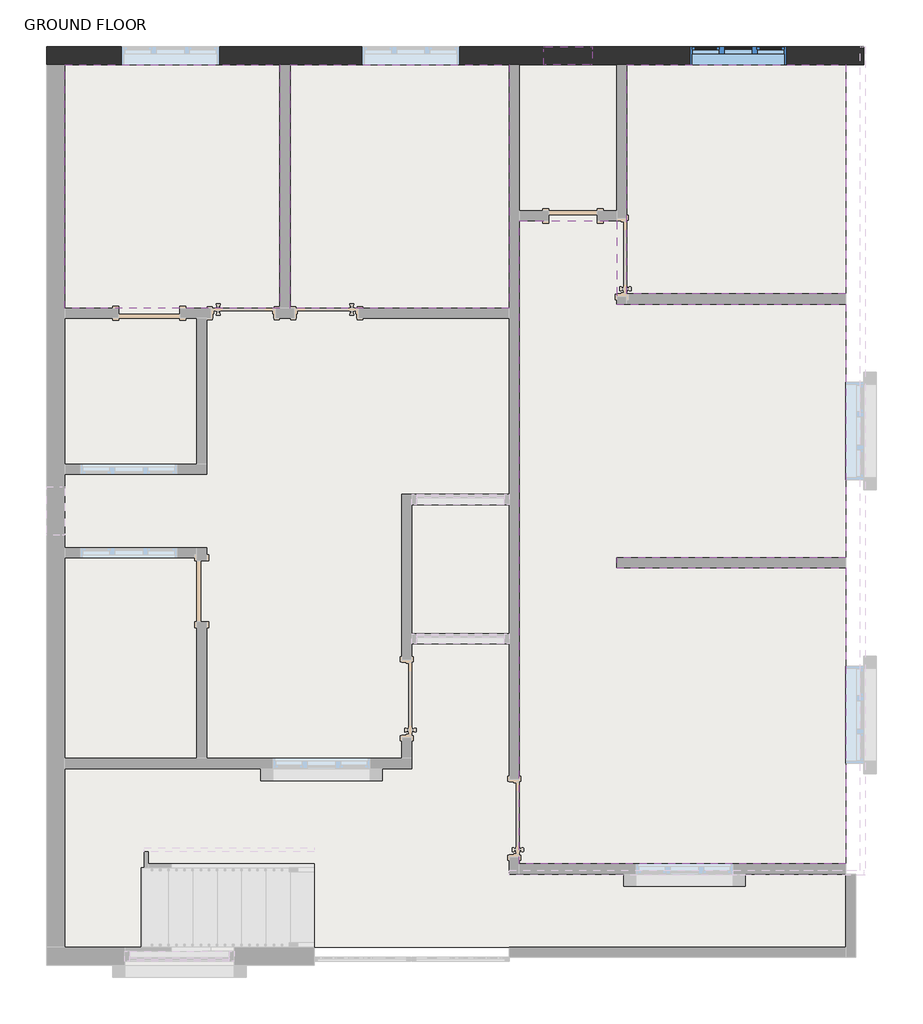
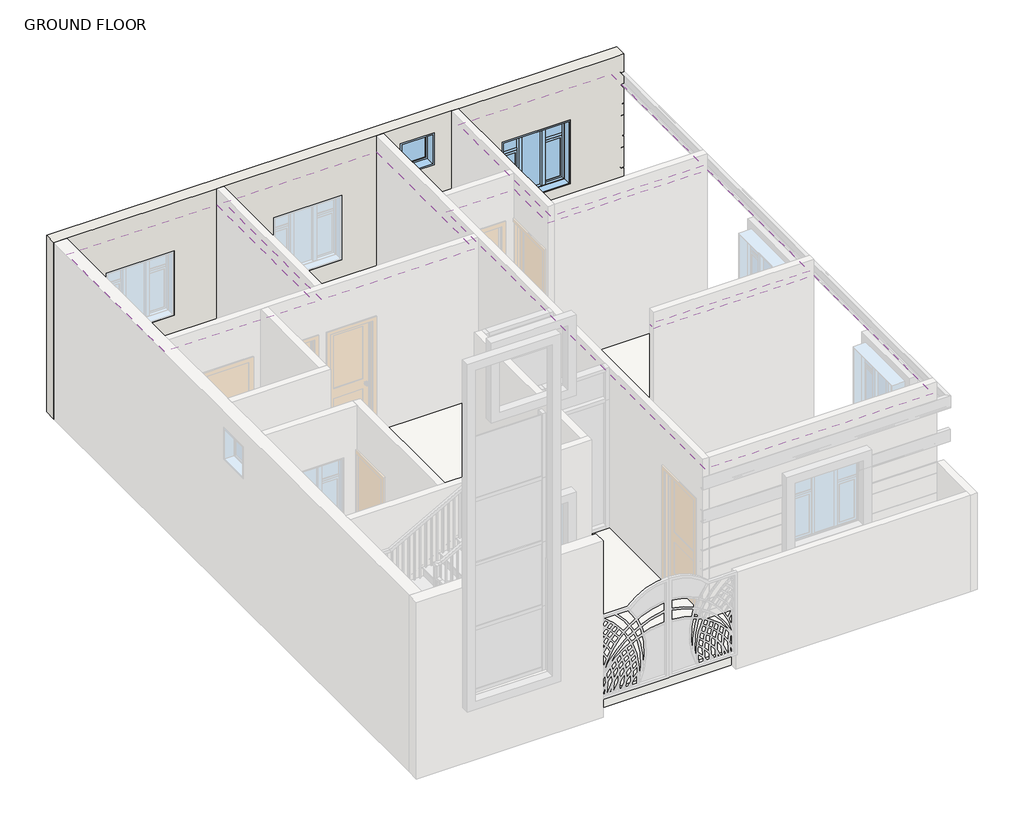
# One storey, part 5 of 7: 4 coverings, 2 windows, 1 slab, 1 wall.
"""IFC4 building model written with IfcOpenShell, lengths in millimetres."""

from ifc_helpers import new_model, si_unit, frame, origin, origin_with_axes, place, context, project, spatial, polyline, circle_curve, outline, extrude, transform, mapped, element, save
from ifc_brep_helpers import plane_surface, cylinder_surface, revolved_surface, advanced_brep
from components import fixed_opening_window_2_x_2_e119d648, window_casement_triple_side_transom_window_4_x_4_fd24aed3

model = new_model("IFC4")

# Units and contexts
model_context = context("Model", 3, world=origin())
ifc_project = project(units=[si_unit("LENGTHUNIT", "METRE", prefix="MILLI")], contexts=[model_context])

# Site, building, storey
site = spatial("IfcSite", under=ifc_project)
building = spatial("IfcBuilding", under=site)
storey = spatial("IfcBuildingStorey", under=building, Name="GROUND FLOOR", Elevation=304.8)

# Coverings
placement = place(None, origin())
element("IfcCovering", 1, ObjectType="GWB on Mtl. Stud 2", at=placement, inside=storey, context=model_context, shape_type="SweptSolid", body=[
    extrude(outline(polyline([(-14760.7023867, 8292.2500137), (-12068.3023867, 8292.2500137), (-12068.3023867, 5244.2500137), (-14760.7023867, 5244.2500137), (-14760.7023867, 8292.2500137)])), frame((0.0, 0.0, 3048.0), z_axis=(0.0, 0.0, 1.0), x_axis=(1.0, 0.0, 0.0)), (0.0, 0.0, 1.0), 107.95),
])
element("IfcCovering", 2, ObjectType="GWB on Mtl. Stud 2", at=placement, inside=storey, context=model_context, shape_type="SweptSolid", body=[
    extrude(outline(polyline([(-11941.3023867, 5244.2500137), (-11941.3023867, 8292.2500137), (-9198.1023867, 8292.2500137), (-9198.1023867, 5244.2500137), (-11941.3023867, 5244.2500137)])), frame((0.0, 0.0, 3048.0), z_axis=(0.0, 0.0, 1.0), x_axis=(1.0, 0.0, 0.0)), (0.0, 0.0, 1.0), 107.95),
])
element("IfcCovering", 3, ObjectType="GWB on Mtl. Stud 2", at=placement, inside=storey, context=model_context, shape_type="SweptSolid", body=[
    extrude(outline(polyline([(-7724.9023867, 5422.0500137), (-7724.9023867, 8292.2500137), (-4981.7023867, 8292.2500137), (-4981.7023867, 5422.0500137), (-7724.9023867, 5422.0500137)])), frame((0.0, 0.0, 3048.0), z_axis=(0.0, 0.0, 1.0), x_axis=(1.0, 0.0, 0.0)), (0.0, 0.0, 1.0), 107.95),
])
element("IfcCovering", 4, ObjectType="GWB on Mtl. Stud 2", at=placement, inside=storey, context=model_context, shape_type="SweptSolid", body=[
    extrude(outline(polyline([(-7851.9023867, 5295.0500137), (-4981.7023867, 5295.0500137), (-4981.7023867, 2120.0500137), (-7851.9023867, 2120.0500137), (-7851.9023867, 1993.0500137), (-4981.7023867, 1993.0500137), (-4981.7023867, -1715.3499863), (-9071.1023867, -1715.3499863), (-9071.1023867, 6336.4500137), (-7851.9023867, 6336.4500137), (-7851.9023867, 5295.0500137)])), frame((0.0, 0.0, 3048.0), z_axis=(0.0, 0.0, 1.0), x_axis=(1.0, 0.0, 0.0)), (0.0, 0.0, 1.0), 107.95),
])

# Slab
element("IfcSlab", 5, ObjectType="FLOORING MARBLE 1'", at=placement, inside=storey, context=model_context, shape_type="SweptSolid", body=[
    extrude(outline(polyline([(-4981.7023867, 8292.2500137), (-4981.7023867, -2756.7499863), (-14760.7023867, -2756.7499863), (-14760.7023867, 8292.2500137), (-4981.7023867, 8292.2500137)])), origin_with_axes(), (0.0, 0.0, 1.0), 304.8),
])

# Wall
element("IfcWall", 6, at=placement, inside=storey, context=model_context, shape_type="AdvancedBrep", body=[
    advanced_brep(
    [(-14990.8898867, 8292.2500137, 0.0), (-14989.3023867, 8292.2500137, 0.0), (-14760.7023867, 8292.2500137, 0.0), (-4981.7023867, 8292.2500137, 0.0), (-4753.1023867, 8292.2500137, 0.0), (-4753.1023867, 8292.2500137, 368.3), (-4801.4639867, 8292.2500137, 368.3), (-4801.4639867, 8292.2500137, 369.6796758), (-4797.0811775, 8292.2500137, 374.8534103), (-4773.4604867, 8292.2500137, 378.7902), (-4754.2226051, 8292.2500137, 381.99652), (-4753.1023867, 8292.2500137, 382.24689), (-4753.1023867, 8292.2500137, 582.95311), (-4754.2226051, 8292.2500137, 583.20348), (-4773.4604867, 8292.2500137, 586.4098), (-4797.0811775, 8292.2500137, 590.3465897), (-4801.4639867, 8292.2500137, 595.5203242), (-4801.4639867, 8292.2500137, 596.9), (-4753.1023867, 8292.2500137, 596.9), (-4753.1023867, 8292.2500137, 977.9), (-4801.4639867, 8292.2500137, 977.9), (-4801.4639867, 8292.2500137, 979.2796758), (-4797.0811775, 8292.2500137, 984.4534103), (-4773.4604867, 8292.2500137, 988.3902), (-4754.2226051, 8292.2500137, 991.59652), (-4753.1023867, 8292.2500137, 991.84689), (-4753.1023867, 8292.2500137, 1192.55311), (-4754.2226051, 8292.2500137, 1192.80348), (-4773.4604867, 8292.2500137, 1196.0098), (-4797.0811775, 8292.2500137, 1199.9465897), (-4801.4639867, 8292.2500137, 1205.1203242), (-4801.4639867, 8292.2500137, 1206.5), (-4753.1023867, 8292.2500137, 1206.5), (-4753.1023867, 8292.2500137, 1587.5), (-4801.4639867, 8292.2500137, 1587.5), (-4801.4639867, 8292.2500137, 1588.8796758), (-4797.0811775, 8292.2500137, 1594.0534103), (-4773.4604867, 8292.2500137, 1597.9902), (-4754.2226051, 8292.2500137, 1601.19652), (-4753.1023867, 8292.2500137, 1601.44689), (-4753.1023867, 8292.2500137, 1802.15311), (-4754.2226051, 8292.2500137, 1802.40348), (-4773.4604867, 8292.2500137, 1805.6098), (-4797.0811775, 8292.2500137, 1809.5465897), (-4801.4639867, 8292.2500137, 1814.7203242), (-4801.4639867, 8292.2500137, 1816.1), (-4753.1023867, 8292.2500137, 1816.1), (-4753.1023867, 8292.2500137, 2197.1), (-4801.4639867, 8292.2500137, 2197.1), (-4801.4639867, 8292.2500137, 2198.4796758), (-4797.0811775, 8292.2500137, 2203.6534103), (-4773.4604867, 8292.2500137, 2207.5902), (-4754.2226051, 8292.2500137, 2210.79652), (-4753.1023867, 8292.2500137, 2211.04689), (-4753.1023867, 8292.2500137, 2411.75311), (-4754.2226051, 8292.2500137, 2412.00348), (-4773.4604867, 8292.2500137, 2415.2098), (-4797.0811775, 8292.2500137, 2419.1465897), (-4801.4639867, 8292.2500137, 2424.3203242), (-4801.4639867, 8292.2500137, 2425.7), (-4753.1023867, 8292.2500137, 2425.7), (-4753.1023867, 8292.2500137, 2781.3), (-4801.4639867, 8292.2500137, 2781.3), (-4801.4639867, 8292.2500137, 2782.6796758), (-4797.0811775, 8292.2500137, 2787.8534103), (-4773.4604867, 8292.2500137, 2791.7902), (-4754.2226051, 8292.2500137, 2794.99652), (-4753.1023867, 8292.2500137, 2795.24689), (-4753.1023867, 8292.2500137, 2995.95311), (-4754.2226051, 8292.2500137, 2996.20348), (-4773.4604867, 8292.2500137, 2999.4098), (-4797.0811775, 8292.2500137, 3003.3465897), (-4801.4639867, 8292.2500137, 3008.5203242), (-4801.4639867, 8292.2500137, 3009.9), (-4753.1023867, 8292.2500137, 3009.9), (-4753.1023867, 8292.2500137, 3352.8), (-4981.7023867, 8292.2500137, 3352.8), (-7724.9023867, 8292.2500137, 3352.8), (-7851.9023867, 8292.2500137, 3352.8), (-9071.1023867, 8292.2500137, 3352.8), (-9198.1023867, 8292.2500137, 3352.8), (-11941.3023867, 8292.2500137, 3352.8), (-12068.3023867, 8292.2500137, 3352.8), (-14760.7023867, 8292.2500137, 3352.8), (-14989.3023867, 8292.2500137, 3352.8), (-14990.8898867, 8292.2500137, 3352.8), (-8156.7023867, 8292.2500137, 3048.0), (-8156.7023867, 8292.2500137, 2438.4), (-8766.3023867, 8292.2500137, 2438.4), (-8766.3023867, 8292.2500137, 3048.0), (-12830.3023867, 8292.2500137, 2438.4), (-12830.3023867, 8292.2500137, 1219.2), (-14049.5023867, 8292.2500137, 1219.2), (-14049.5023867, 8292.2500137, 2438.4), (-9820.4023867, 8292.2500137, 2438.4), (-9820.4023867, 8292.2500137, 1219.2), (-11039.6023867, 8292.2500137, 1219.2), (-11039.6023867, 8292.2500137, 2438.4), (-5718.3023867, 8292.2500137, 2438.4), (-5718.3023867, 8292.2500137, 1219.2), (-6937.5023867, 8292.2500137, 1219.2), (-6937.5023867, 8292.2500137, 2438.4), (-4753.1023867, 8520.8500137, 0.0), (-14990.8898867, 8520.8500137, 0.0), (-14990.8898867, 8520.8500137, 3352.8), (-4753.1023867, 8520.8500137, 3352.8), (-4753.1023867, 8520.8500137, 3009.9), (-4801.4639867, 8520.8500137, 3009.9), (-4801.4639867, 8520.8500137, 3008.5203242), (-4797.0811775, 8520.8500137, 3003.3465897), (-4773.4604867, 8520.8500137, 2999.4098), (-4754.2226051, 8520.8500137, 2996.20348), (-4753.1023867, 8520.8500137, 2995.95311), (-4753.1023867, 8520.8500137, 2795.24689), (-4754.2226051, 8520.8500137, 2794.99652), (-4773.4604867, 8520.8500137, 2791.7902), (-4797.0811775, 8520.8500137, 2787.8534103), (-4801.4639867, 8520.8500137, 2782.6796758), (-4801.4639867, 8520.8500137, 2781.3), (-4753.1023867, 8520.8500137, 2781.3), (-4753.1023867, 8520.8500137, 2425.7), (-4801.4639867, 8520.8500137, 2425.7), (-4801.4639867, 8520.8500137, 2424.3203242), (-4797.0811775, 8520.8500137, 2419.1465897), (-4773.4604867, 8520.8500137, 2415.2098), (-4754.2226051, 8520.8500137, 2412.00348), (-4753.1023867, 8520.8500137, 2411.75311), (-4753.1023867, 8520.8500137, 2211.04689), (-4754.2226051, 8520.8500137, 2210.79652), (-4773.4604867, 8520.8500137, 2207.5902), (-4797.0811775, 8520.8500137, 2203.6534103), (-4801.4639867, 8520.8500137, 2198.4796758), (-4801.4639867, 8520.8500137, 2197.1), (-4753.1023867, 8520.8500137, 2197.1), (-4753.1023867, 8520.8500137, 1816.1), (-4801.4639867, 8520.8500137, 1816.1), (-4801.4639867, 8520.8500137, 1814.7203242), (-4797.0811775, 8520.8500137, 1809.5465897), (-4773.4604867, 8520.8500137, 1805.6098), (-4754.2226051, 8520.8500137, 1802.40348), (-4753.1023867, 8520.8500137, 1802.15311), (-4753.1023867, 8520.8500137, 1601.44689), (-4754.2226051, 8520.8500137, 1601.19652), (-4773.4604867, 8520.8500137, 1597.9902), (-4797.0811775, 8520.8500137, 1594.0534103), (-4801.4639867, 8520.8500137, 1588.8796758), (-4801.4639867, 8520.8500137, 1587.5), (-4753.1023867, 8520.8500137, 1587.5), (-4753.1023867, 8520.8500137, 1206.5), (-4801.4639867, 8520.8500137, 1206.5), (-4801.4639867, 8520.8500137, 1205.1203242), (-4797.0811775, 8520.8500137, 1199.9465897), (-4773.4604867, 8520.8500137, 1196.0098), (-4754.2226051, 8520.8500137, 1192.80348), (-4753.1023867, 8520.8500137, 1192.55311), (-4753.1023867, 8520.8500137, 991.84689), (-4754.2226051, 8520.8500137, 991.59652), (-4773.4604867, 8520.8500137, 988.3902), (-4797.0811775, 8520.8500137, 984.4534103), (-4801.4639867, 8520.8500137, 979.2796758), (-4801.4639867, 8520.8500137, 977.9), (-4753.1023867, 8520.8500137, 977.9), (-4753.1023867, 8520.8500137, 596.9), (-4801.4639867, 8520.8500137, 596.9), (-4801.4639867, 8520.8500137, 595.5203242), (-4797.0811775, 8520.8500137, 590.3465897), (-4773.4604867, 8520.8500137, 586.4098), (-4754.2226051, 8520.8500137, 583.20348), (-4753.1023867, 8520.8500137, 582.95311), (-4753.1023867, 8520.8500137, 382.24689), (-4754.2226051, 8520.8500137, 381.99652), (-4773.4604867, 8520.8500137, 378.7902), (-4797.0811775, 8520.8500137, 374.8534103), (-4801.4639867, 8520.8500137, 369.6796758), (-4801.4639867, 8520.8500137, 368.3), (-4753.1023867, 8520.8500137, 368.3), (-8156.7023867, 8520.8500137, 2438.4), (-8156.7023867, 8520.8500137, 3048.0), (-8766.3023867, 8520.8500137, 3048.0), (-8766.3023867, 8520.8500137, 2438.4), (-12830.3023867, 8520.8500137, 1219.2), (-12830.3023867, 8520.8500137, 2438.4), (-14049.5023867, 8520.8500137, 2438.4), (-14049.5023867, 8520.8500137, 1219.2), (-9820.4023867, 8520.8500137, 1219.2), (-9820.4023867, 8520.8500137, 2438.4), (-11039.6023867, 8520.8500137, 2438.4), (-11039.6023867, 8520.8500137, 1219.2), (-5718.3023867, 8520.8500137, 1219.2), (-5718.3023867, 8520.8500137, 2438.4), (-6937.5023867, 8520.8500137, 2438.4), (-6937.5023867, 8520.8500137, 1219.2)],
    [
        (0, 1),
        (1, 2),
        (2, 3),
        (3, 4),
        (4, 5),
        (5, 6),
        (6, 7),
        (7, 8, circle_curve(frame((-4796.2188867, 8292.2500137, 369.6796758), z_axis=(0.0, 1.0, 0.0), x_axis=(-1.0, 0.0, 0.0)), 5.2451)),
        (8, 9),
        (9, 10),
        (10, 11, circle_curve(frame((-4755.9471867, 8292.2500137, 392.343989), z_axis=(0.0, -1.0, 0.0), x_axis=(-1.0, 0.0, 0.0)), 10.4902)),
        (11, 12),
        (12, 13, circle_curve(frame((-4755.9471867, 8292.2500137, 572.856011), z_axis=(0.0, -1.0, 0.0), x_axis=(-1.0, 0.0, 0.0)), 10.4902)),
        (13, 14),
        (14, 15),
        (15, 16, circle_curve(frame((-4796.2188867, 8292.2500137, 595.5203242), z_axis=(0.0, 1.0, 0.0), x_axis=(-1.0, 0.0, 0.0)), 5.2451)),
        (16, 17),
        (17, 18),
        (18, 19),
        (19, 20),
        (20, 21),
        (21, 22, circle_curve(frame((-4796.2188867, 8292.2500137, 979.2796758), z_axis=(0.0, 1.0, 0.0), x_axis=(-1.0, 0.0, 0.0)), 5.2451)),
        (22, 23),
        (23, 24),
        (24, 25, circle_curve(frame((-4755.9471867, 8292.2500137, 1001.943989), z_axis=(0.0, -1.0, 0.0), x_axis=(-1.0, 0.0, 0.0)), 10.4902)),
        (25, 26),
        (26, 27, circle_curve(frame((-4755.9471867, 8292.2500137, 1182.456011), z_axis=(0.0, -1.0, 0.0), x_axis=(-1.0, 0.0, 0.0)), 10.4902)),
        (27, 28),
        (28, 29),
        (29, 30, circle_curve(frame((-4796.2188867, 8292.2500137, 1205.1203242), z_axis=(0.0, 1.0, 0.0), x_axis=(-1.0, 0.0, 0.0)), 5.2451)),
        (30, 31),
        (31, 32),
        (32, 33),
        (33, 34),
        (34, 35),
        (35, 36, circle_curve(frame((-4796.2188867, 8292.2500137, 1588.8796758), z_axis=(0.0, 1.0, 0.0), x_axis=(-1.0, 0.0, 0.0)), 5.2451)),
        (36, 37),
        (37, 38),
        (38, 39, circle_curve(frame((-4755.9471867, 8292.2500137, 1611.543989), z_axis=(0.0, -1.0, 0.0), x_axis=(-1.0, 0.0, 0.0)), 10.4902)),
        (39, 40),
        (40, 41, circle_curve(frame((-4755.9471867, 8292.2500137, 1792.056011), z_axis=(0.0, -1.0, 0.0), x_axis=(-1.0, 0.0, 0.0)), 10.4902)),
        (41, 42),
        (42, 43),
        (43, 44, circle_curve(frame((-4796.2188867, 8292.2500137, 1814.7203242), z_axis=(0.0, 1.0, 0.0), x_axis=(-1.0, 0.0, 0.0)), 5.2451)),
        (44, 45),
        (45, 46),
        (46, 47),
        (47, 48),
        (48, 49),
        (49, 50, circle_curve(frame((-4796.2188867, 8292.2500137, 2198.4796758), z_axis=(0.0, 1.0, 0.0), x_axis=(-1.0, 0.0, 0.0)), 5.2451)),
        (50, 51),
        (51, 52),
        (52, 53, circle_curve(frame((-4755.9471867, 8292.2500137, 2221.143989), z_axis=(0.0, -1.0, 0.0), x_axis=(-1.0, 0.0, 0.0)), 10.4902)),
        (53, 54),
        (54, 55, circle_curve(frame((-4755.9471867, 8292.2500137, 2401.656011), z_axis=(0.0, -1.0, 0.0), x_axis=(-1.0, 0.0, 0.0)), 10.4902)),
        (55, 56),
        (56, 57),
        (57, 58, circle_curve(frame((-4796.2188867, 8292.2500137, 2424.3203242), z_axis=(0.0, 1.0, 0.0), x_axis=(-1.0, 0.0, 0.0)), 5.2451)),
        (58, 59),
        (59, 60),
        (60, 61),
        (61, 62),
        (62, 63),
        (63, 64, circle_curve(frame((-4796.2188867, 8292.2500137, 2782.6796758), z_axis=(0.0, 1.0, 0.0), x_axis=(-1.0, 0.0, 0.0)), 5.2451)),
        (64, 65),
        (65, 66),
        (66, 67, circle_curve(frame((-4755.9471867, 8292.2500137, 2805.343989), z_axis=(0.0, -1.0, 0.0), x_axis=(-1.0, 0.0, 0.0)), 10.4902)),
        (67, 68),
        (68, 69, circle_curve(frame((-4755.9471867, 8292.2500137, 2985.856011), z_axis=(0.0, -1.0, 0.0), x_axis=(-1.0, 0.0, 0.0)), 10.4902)),
        (69, 70),
        (70, 71),
        (71, 72, circle_curve(frame((-4796.2188867, 8292.2500137, 3008.5203242), z_axis=(0.0, 1.0, 0.0), x_axis=(-1.0, 0.0, 0.0)), 5.2451)),
        (72, 73),
        (73, 74),
        (74, 75),
        (75, 76),
        (76, 77),
        (77, 78),
        (78, 79),
        (79, 80),
        (80, 81),
        (81, 82),
        (82, 83),
        (83, 84),
        (84, 85),
        (85, 0),
        (86, 87),
        (87, 88),
        (88, 89),
        (89, 86),
        (90, 91),
        (91, 92),
        (92, 93),
        (93, 90),
        (94, 95),
        (95, 96),
        (96, 97),
        (97, 94),
        (98, 99),
        (99, 100),
        (100, 101),
        (101, 98),
        (102, 103),
        (103, 104),
        (104, 105),
        (105, 106),
        (106, 107),
        (107, 108),
        (108, 109, circle_curve(frame((-4796.2188867, 8520.8500137, 3008.5203242), z_axis=(0.0, -1.0, 0.0), x_axis=(-1.0, 0.0, 0.0)), 5.2451)),
        (109, 110),
        (110, 111),
        (111, 112, circle_curve(frame((-4755.9471867, 8520.8500137, 2985.856011), z_axis=(0.0, 1.0, 0.0), x_axis=(-1.0, 0.0, 0.0)), 10.4902)),
        (112, 113),
        (113, 114, circle_curve(frame((-4755.9471867, 8520.8500137, 2805.343989), z_axis=(0.0, 1.0, 0.0), x_axis=(-1.0, 0.0, 0.0)), 10.4902)),
        (114, 115),
        (115, 116),
        (116, 117, circle_curve(frame((-4796.2188867, 8520.8500137, 2782.6796758), z_axis=(0.0, -1.0, 0.0), x_axis=(-1.0, 0.0, 0.0)), 5.2451)),
        (117, 118),
        (118, 119),
        (119, 120),
        (120, 121),
        (121, 122),
        (122, 123, circle_curve(frame((-4796.2188867, 8520.8500137, 2424.3203242), z_axis=(0.0, -1.0, 0.0), x_axis=(-1.0, 0.0, 0.0)), 5.2451)),
        (123, 124),
        (124, 125),
        (125, 126, circle_curve(frame((-4755.9471867, 8520.8500137, 2401.656011), z_axis=(0.0, 1.0, 0.0), x_axis=(-1.0, 0.0, 0.0)), 10.4902)),
        (126, 127),
        (127, 128, circle_curve(frame((-4755.9471867, 8520.8500137, 2221.143989), z_axis=(0.0, 1.0, 0.0), x_axis=(-1.0, 0.0, 0.0)), 10.4902)),
        (128, 129),
        (129, 130),
        (130, 131, circle_curve(frame((-4796.2188867, 8520.8500137, 2198.4796758), z_axis=(0.0, -1.0, 0.0), x_axis=(-1.0, 0.0, 0.0)), 5.2451)),
        (131, 132),
        (132, 133),
        (133, 134),
        (134, 135),
        (135, 136),
        (136, 137, circle_curve(frame((-4796.2188867, 8520.8500137, 1814.7203242), z_axis=(0.0, -1.0, 0.0), x_axis=(-1.0, 0.0, 0.0)), 5.2451)),
        (137, 138),
        (138, 139),
        (139, 140, circle_curve(frame((-4755.9471867, 8520.8500137, 1792.056011), z_axis=(0.0, 1.0, 0.0), x_axis=(-1.0, 0.0, 0.0)), 10.4902)),
        (140, 141),
        (141, 142, circle_curve(frame((-4755.9471867, 8520.8500137, 1611.543989), z_axis=(0.0, 1.0, 0.0), x_axis=(-1.0, 0.0, 0.0)), 10.4902)),
        (142, 143),
        (143, 144),
        (144, 145, circle_curve(frame((-4796.2188867, 8520.8500137, 1588.8796758), z_axis=(0.0, -1.0, 0.0), x_axis=(-1.0, 0.0, 0.0)), 5.2451)),
        (145, 146),
        (146, 147),
        (147, 148),
        (148, 149),
        (149, 150),
        (150, 151, circle_curve(frame((-4796.2188867, 8520.8500137, 1205.1203242), z_axis=(0.0, -1.0, 0.0), x_axis=(-1.0, 0.0, 0.0)), 5.2451)),
        (151, 152),
        (152, 153),
        (153, 154, circle_curve(frame((-4755.9471867, 8520.8500137, 1182.456011), z_axis=(0.0, 1.0, 0.0), x_axis=(-1.0, 0.0, 0.0)), 10.4902)),
        (154, 155),
        (155, 156, circle_curve(frame((-4755.9471867, 8520.8500137, 1001.943989), z_axis=(0.0, 1.0, 0.0), x_axis=(-1.0, 0.0, 0.0)), 10.4902)),
        (156, 157),
        (157, 158),
        (158, 159, circle_curve(frame((-4796.2188867, 8520.8500137, 979.2796758), z_axis=(0.0, -1.0, 0.0), x_axis=(-1.0, 0.0, 0.0)), 5.2451)),
        (159, 160),
        (160, 161),
        (161, 162),
        (162, 163),
        (163, 164),
        (164, 165, circle_curve(frame((-4796.2188867, 8520.8500137, 595.5203242), z_axis=(0.0, -1.0, 0.0), x_axis=(-1.0, 0.0, 0.0)), 5.2451)),
        (165, 166),
        (166, 167),
        (167, 168, circle_curve(frame((-4755.9471867, 8520.8500137, 572.856011), z_axis=(0.0, 1.0, 0.0), x_axis=(-1.0, 0.0, 0.0)), 10.4902)),
        (168, 169),
        (169, 170, circle_curve(frame((-4755.9471867, 8520.8500137, 392.343989), z_axis=(0.0, 1.0, 0.0), x_axis=(-1.0, 0.0, 0.0)), 10.4902)),
        (170, 171),
        (171, 172),
        (172, 173, circle_curve(frame((-4796.2188867, 8520.8500137, 369.6796758), z_axis=(0.0, -1.0, 0.0), x_axis=(-1.0, 0.0, 0.0)), 5.2451)),
        (173, 174),
        (174, 175),
        (175, 102),
        (176, 177),
        (177, 178),
        (178, 179),
        (179, 176),
        (180, 181),
        (181, 182),
        (182, 183),
        (183, 180),
        (184, 185),
        (185, 186),
        (186, 187),
        (187, 184),
        (188, 189),
        (189, 190),
        (190, 191),
        (191, 188),
        (0, 103),
        (102, 4),
        (75, 105),
        (104, 85),
        (175, 5),
        (74, 106),
        (67, 113),
        (112, 68),
        (119, 61),
        (60, 120),
        (133, 47),
        (46, 134),
        (53, 127),
        (126, 54),
        (147, 33),
        (32, 148),
        (39, 141),
        (140, 40),
        (18, 162),
        (161, 19),
        (11, 169),
        (168, 12),
        (25, 155),
        (154, 26),
        (176, 87),
        (86, 177),
        (179, 88),
        (178, 89),
        (90, 181),
        (180, 91),
        (183, 92),
        (182, 93),
        (94, 185),
        (184, 95),
        (187, 96),
        (186, 97),
        (98, 189),
        (188, 99),
        (191, 100),
        (190, 101),
        (118, 62),
        (117, 63),
        (116, 64),
        (115, 65),
        (114, 66),
        (111, 69),
        (110, 70),
        (109, 71),
        (108, 72),
        (107, 73),
        (132, 48),
        (131, 49),
        (130, 50),
        (129, 51),
        (128, 52),
        (125, 55),
        (124, 56),
        (123, 57),
        (122, 58),
        (121, 59),
        (146, 34),
        (145, 35),
        (144, 36),
        (143, 37),
        (142, 38),
        (139, 41),
        (138, 42),
        (137, 43),
        (136, 44),
        (135, 45),
        (174, 6),
        (173, 7),
        (172, 8),
        (171, 9),
        (170, 10),
        (167, 13),
        (166, 14),
        (165, 15),
        (164, 16),
        (163, 17),
        (160, 20),
        (159, 21),
        (158, 22),
        (157, 23),
        (156, 24),
        (153, 27),
        (152, 28),
        (151, 29),
        (150, 30),
        (149, 31),
    ],
    [
        plane_surface(frame((-14983.6015581, 8292.2500137, 0.0), z_axis=(0.0, -1.0, 0.0), x_axis=(1.0, 0.0, 0.0))),
        plane_surface(frame((-14983.6015581, 8520.8500137, 0.0), z_axis=(0.0, 1.0, 0.0), x_axis=(-1.0, 0.0, 0.0))),
        plane_surface(frame((-14990.8898867, 8292.2500137, 0.0), z_axis=(0.0, 0.0, -1.0), x_axis=(0.0, 1.0, 0.0))),
        plane_surface(frame((-4867.4023867, 8292.2500137, 3352.8), z_axis=(0.0, 0.0, 1.0), x_axis=(0.0, 1.0, 0.0))),
        plane_surface(frame((-14990.8898867, 8292.2500137, 3352.8), z_axis=(-1.0, 0.0, 0.0), x_axis=(0.0, 1.0, 0.0))),
        plane_surface(frame((-4753.1023867, 8520.8500137, 0.0), z_axis=(1.0, 0.0, 0.0), x_axis=(0.0, 1.0, 0.0))),
        plane_surface(frame((-8156.7023867, 9816.2500137, 3048.0), z_axis=(-1.0, 0.0, 0.0), x_axis=(0.0, -1.0, 0.0))),
        plane_surface(frame((-8156.7023867, 9816.2500137, 2438.4), z_axis=(0.0, 0.0, 1.0), x_axis=(0.0, -1.0, 0.0))),
        plane_surface(frame((-8766.3023867, 9816.2500137, 2438.4), z_axis=(1.0, 0.0, 0.0), x_axis=(0.0, -1.0, 0.0))),
        plane_surface(frame((-8766.3023867, 9816.2500137, 3048.0), z_axis=(0.0, 0.0, -1.0), x_axis=(0.0, -1.0, 0.0))),
        plane_surface(frame((-12830.3023867, 8292.2500137, 2438.4), z_axis=(-1.0, 0.0, 0.0), x_axis=(0.0, 1.0, 0.0))),
        plane_surface(frame((-12830.3023867, 8292.2500137, 1219.2), z_axis=(0.0, 0.0, 1.0), x_axis=(0.0, 1.0, 0.0))),
        plane_surface(frame((-14049.5023867, 8292.2500137, 1219.2), z_axis=(1.0, 0.0, 0.0), x_axis=(0.0, 1.0, 0.0))),
        plane_surface(frame((-14049.5023867, 8292.2500137, 2438.4), z_axis=(0.0, 0.0, -1.0), x_axis=(0.0, 1.0, 0.0))),
        plane_surface(frame((-9820.4023867, 8292.2500137, 2438.4), z_axis=(-1.0, 0.0, 0.0), x_axis=(0.0, 1.0, 0.0))),
        plane_surface(frame((-9820.4023867, 8292.2500137, 1219.2), z_axis=(0.0, 0.0, 1.0), x_axis=(0.0, 1.0, 0.0))),
        plane_surface(frame((-11039.6023867, 8292.2500137, 1219.2), z_axis=(1.0, 0.0, 0.0), x_axis=(0.0, 1.0, 0.0))),
        plane_surface(frame((-11039.6023867, 8292.2500137, 2438.4), z_axis=(0.0, 0.0, -1.0), x_axis=(0.0, 1.0, 0.0))),
        plane_surface(frame((-5718.3023867, 8292.2500137, 2438.4), z_axis=(-1.0, 0.0, 0.0), x_axis=(0.0, 1.0, 0.0))),
        plane_surface(frame((-5718.3023867, 8292.2500137, 1219.2), z_axis=(0.0, 0.0, 1.0), x_axis=(0.0, 1.0, 0.0))),
        plane_surface(frame((-6937.5023867, 8292.2500137, 1219.2), z_axis=(1.0, 0.0, 0.0), x_axis=(0.0, 1.0, 0.0))),
        plane_surface(frame((-6937.5023867, 8292.2500137, 2438.4), z_axis=(0.0, 0.0, -1.0), x_axis=(0.0, 1.0, 0.0))),
        plane_surface(frame((-4738.2179867, 8520.8500137, 2781.3), z_axis=(0.0, 0.0, 1.0), x_axis=(0.0, -1.0, 0.0))),
        plane_surface(frame((-4801.4639867, 8520.8500137, 2781.3), z_axis=(1.0, 0.0, 0.0), x_axis=(0.0, -1.0, 0.0))),
        revolved_surface(polyline([(-4801.4639867000005, 8520.8500137, 2782.6796758), (-4801.4639867000005, 8292.2500137, 2782.6796758)]), (-4796.2188867, 8520.8500137, 2782.6796758), (0.0, 1.0, 0.0)),
        plane_surface(frame((-4797.0811775, 8520.8500137, 2787.8534103), z_axis=(0.16439930721687793, 0.0, -0.9863938705135037), x_axis=(0.0, -1.0, 0.0))),
        plane_surface(frame((-4773.4604867, 8520.8500137, 2791.7902), z_axis=(0.1643993072168769, 0.0, -0.9863938705135039), x_axis=(0.0, -1.0, 0.0))),
        cylinder_surface(frame((-4755.9471867, 8520.8500137, 2805.343989), z_axis=(0.0, -1.0, 0.0), x_axis=(-1.0, 0.0, 0.0)), 10.4902),
        cylinder_surface(frame((-4755.9471867, 8520.8500137, 2985.856011), z_axis=(0.0, -1.0, 0.0), x_axis=(-1.0, 0.0, 0.0)), 10.4902),
        plane_surface(frame((-4754.2226051, 8520.8500137, 2996.20348), z_axis=(0.16439930721687146, 0.0, 0.9863938705135048), x_axis=(0.0, -1.0, 0.0))),
        plane_surface(frame((-4773.4604867, 8520.8500137, 2999.4098), z_axis=(0.16439930721687082, 0.0, 0.9863938705135049), x_axis=(0.0, -1.0, 0.0))),
        revolved_surface(polyline([(-4801.4639867000005, 8520.8500137, 3008.5203242), (-4801.4639867000005, 8292.2500137, 3008.5203242)]), (-4796.2188867, 8520.8500137, 3008.5203242), (0.0, 1.0, 0.0)),
        plane_surface(frame((-4801.4639867, 8520.8500137, 3008.5203242), z_axis=(1.0, 0.0, 0.0), x_axis=(0.0, -1.0, 0.0))),
        plane_surface(frame((-4801.4639867, 8520.8500137, 3009.9), z_axis=(0.0, 0.0, -1.0), x_axis=(0.0, -1.0, 0.0))),
        plane_surface(frame((-4738.2179867, 8520.8500137, 2197.1), z_axis=(0.0, 0.0, 1.0), x_axis=(0.0, -1.0, 0.0))),
        plane_surface(frame((-4801.4639867, 8520.8500137, 2197.1), z_axis=(1.0, 0.0, 0.0), x_axis=(0.0, -1.0, 0.0))),
        revolved_surface(polyline([(-4801.4639867000005, 8520.8500137, 2198.4796758), (-4801.4639867000005, 8292.2500137, 2198.4796758)]), (-4796.2188867, 8520.8500137, 2198.4796758), (0.0, 1.0, 0.0)),
        plane_surface(frame((-4797.0811775, 8520.8500137, 2203.6534103), z_axis=(0.16439930721687793, 0.0, -0.9863938705135037), x_axis=(0.0, -1.0, 0.0))),
        plane_surface(frame((-4773.4604867, 8520.8500137, 2207.5902), z_axis=(0.1643993072168769, 0.0, -0.9863938705135039), x_axis=(0.0, -1.0, 0.0))),
        cylinder_surface(frame((-4755.9471867, 8520.8500137, 2221.143989), z_axis=(0.0, -1.0, 0.0), x_axis=(-1.0, 0.0, 0.0)), 10.4902),
        cylinder_surface(frame((-4755.9471867, 8520.8500137, 2401.656011), z_axis=(0.0, -1.0, 0.0), x_axis=(-1.0, 0.0, 0.0)), 10.4902),
        plane_surface(frame((-4754.2226051, 8520.8500137, 2412.00348), z_axis=(0.16439930721687146, 0.0, 0.9863938705135048), x_axis=(0.0, -1.0, 0.0))),
        plane_surface(frame((-4773.4604867, 8520.8500137, 2415.2098), z_axis=(0.16439930721687082, 0.0, 0.9863938705135049), x_axis=(0.0, -1.0, 0.0))),
        revolved_surface(polyline([(-4801.4639867000005, 8520.8500137, 2424.3203242), (-4801.4639867000005, 8292.2500137, 2424.3203242)]), (-4796.2188867, 8520.8500137, 2424.3203242), (0.0, 1.0, 0.0)),
        plane_surface(frame((-4801.4639867, 8520.8500137, 2424.3203242), z_axis=(1.0, 0.0, 0.0), x_axis=(0.0, -1.0, 0.0))),
        plane_surface(frame((-4801.4639867, 8520.8500137, 2425.7), z_axis=(0.0, 0.0, -1.0), x_axis=(0.0, -1.0, 0.0))),
        plane_surface(frame((-4738.2179867, 8520.8500137, 1587.5), z_axis=(0.0, 0.0, 1.0), x_axis=(0.0, -1.0, 0.0))),
        plane_surface(frame((-4801.4639867, 8520.8500137, 1587.5), z_axis=(1.0, 0.0, 0.0), x_axis=(0.0, -1.0, 0.0))),
        revolved_surface(polyline([(-4801.4639867000005, 8520.8500137, 1588.8796758), (-4801.4639867000005, 8292.2500137, 1588.8796758)]), (-4796.2188867, 8520.8500137, 1588.8796758), (0.0, 1.0, 0.0)),
        plane_surface(frame((-4797.0811775, 8520.8500137, 1594.0534103), z_axis=(0.16439930721687793, 0.0, -0.9863938705135037), x_axis=(0.0, -1.0, 0.0))),
        plane_surface(frame((-4773.4604867, 8520.8500137, 1597.9902), z_axis=(0.1643993072168769, 0.0, -0.9863938705135039), x_axis=(0.0, -1.0, 0.0))),
        cylinder_surface(frame((-4755.9471867, 8520.8500137, 1611.543989), z_axis=(0.0, -1.0, 0.0), x_axis=(-1.0, 0.0, 0.0)), 10.4902),
        cylinder_surface(frame((-4755.9471867, 8520.8500137, 1792.056011), z_axis=(0.0, -1.0, 0.0), x_axis=(-1.0, 0.0, 0.0)), 10.4902),
        plane_surface(frame((-4754.2226051, 8520.8500137, 1802.40348), z_axis=(0.16439930721687146, 0.0, 0.9863938705135048), x_axis=(0.0, -1.0, 0.0))),
        plane_surface(frame((-4773.4604867, 8520.8500137, 1805.6098), z_axis=(0.16439930721687082, 0.0, 0.9863938705135049), x_axis=(0.0, -1.0, 0.0))),
        revolved_surface(polyline([(-4801.4639867000005, 8520.8500137, 1814.7203242), (-4801.4639867000005, 8292.2500137, 1814.7203242)]), (-4796.2188867, 8520.8500137, 1814.7203242), (0.0, 1.0, 0.0)),
        plane_surface(frame((-4801.4639867, 8520.8500137, 1814.7203242), z_axis=(1.0, 0.0, 0.0), x_axis=(0.0, -1.0, 0.0))),
        plane_surface(frame((-4801.4639867, 8520.8500137, 1816.1), z_axis=(0.0, 0.0, -1.0), x_axis=(0.0, -1.0, 0.0))),
        plane_surface(frame((-4738.2179867, 8520.8500137, 368.3), z_axis=(0.0, 0.0, 1.0), x_axis=(0.0, -1.0, 0.0))),
        plane_surface(frame((-4801.4639867, 8520.8500137, 368.3), z_axis=(1.0, 0.0, 0.0), x_axis=(0.0, -1.0, 0.0))),
        revolved_surface(polyline([(-4801.4639867000005, 8520.8500137, 369.6796758), (-4801.4639867000005, 8292.2500137, 369.6796758)]), (-4796.2188867, 8520.8500137, 369.6796758), (0.0, 1.0, 0.0)),
        plane_surface(frame((-4797.0811775, 8520.8500137, 374.8534103), z_axis=(0.16439930721687793, 0.0, -0.9863938705135037), x_axis=(0.0, -1.0, 0.0))),
        plane_surface(frame((-4773.4604867, 8520.8500137, 378.7902), z_axis=(0.1643993072168769, 0.0, -0.9863938705135039), x_axis=(0.0, -1.0, 0.0))),
        cylinder_surface(frame((-4755.9471867, 8520.8500137, 392.343989), z_axis=(0.0, -1.0, 0.0), x_axis=(-1.0, 0.0, 0.0)), 10.4902),
        cylinder_surface(frame((-4755.9471867, 8520.8500137, 572.856011), z_axis=(0.0, -1.0, 0.0), x_axis=(-1.0, 0.0, 0.0)), 10.4902),
        plane_surface(frame((-4754.2226051, 8520.8500137, 583.20348), z_axis=(0.16439930721687146, 0.0, 0.9863938705135048), x_axis=(0.0, -1.0, 0.0))),
        plane_surface(frame((-4773.4604867, 8520.8500137, 586.4098), z_axis=(0.16439930721687082, 0.0, 0.9863938705135049), x_axis=(0.0, -1.0, 0.0))),
        revolved_surface(polyline([(-4801.4639867000005, 8520.8500137, 595.5203242), (-4801.4639867000005, 8292.2500137, 595.5203242)]), (-4796.2188867, 8520.8500137, 595.5203242), (0.0, 1.0, 0.0)),
        plane_surface(frame((-4801.4639867, 8520.8500137, 595.5203242), z_axis=(1.0, 0.0, 0.0), x_axis=(0.0, -1.0, 0.0))),
        plane_surface(frame((-4801.4639867, 8520.8500137, 596.9), z_axis=(0.0, 0.0, -1.0), x_axis=(0.0, -1.0, 0.0))),
        plane_surface(frame((-4738.2179867, 8520.8500137, 977.9), z_axis=(0.0, 0.0, 1.0), x_axis=(0.0, -1.0, 0.0))),
        plane_surface(frame((-4801.4639867, 8520.8500137, 977.9), z_axis=(1.0, 0.0, 0.0), x_axis=(0.0, -1.0, 0.0))),
        revolved_surface(polyline([(-4801.4639867000005, 8520.8500137, 979.2796758), (-4801.4639867000005, 8292.2500137, 979.2796758)]), (-4796.2188867, 8520.8500137, 979.2796758), (0.0, 1.0, 0.0)),
        plane_surface(frame((-4797.0811775, 8520.8500137, 984.4534103), z_axis=(0.16439930721687793, 0.0, -0.9863938705135037), x_axis=(0.0, -1.0, 0.0))),
        plane_surface(frame((-4773.4604867, 8520.8500137, 988.3902), z_axis=(0.1643993072168769, 0.0, -0.9863938705135039), x_axis=(0.0, -1.0, 0.0))),
        cylinder_surface(frame((-4755.9471867, 8520.8500137, 1001.943989), z_axis=(0.0, -1.0, 0.0), x_axis=(-1.0, 0.0, 0.0)), 10.4902),
        cylinder_surface(frame((-4755.9471867, 8520.8500137, 1182.456011), z_axis=(0.0, -1.0, 0.0), x_axis=(-1.0, 0.0, 0.0)), 10.4902),
        plane_surface(frame((-4754.2226051, 8520.8500137, 1192.80348), z_axis=(0.16439930721687146, 0.0, 0.9863938705135048), x_axis=(0.0, -1.0, 0.0))),
        plane_surface(frame((-4773.4604867, 8520.8500137, 1196.0098), z_axis=(0.16439930721687082, 0.0, 0.9863938705135049), x_axis=(0.0, -1.0, 0.0))),
        revolved_surface(polyline([(-4801.4639867000005, 8520.8500137, 1205.1203242), (-4801.4639867000005, 8292.2500137, 1205.1203242)]), (-4796.2188867, 8520.8500137, 1205.1203242), (0.0, 1.0, 0.0)),
        plane_surface(frame((-4801.4639867, 8520.8500137, 1205.1203242), z_axis=(1.0, 0.0, 0.0), x_axis=(0.0, -1.0, 0.0))),
        plane_surface(frame((-4801.4639867, 8520.8500137, 1206.5), z_axis=(0.0, 0.0, -1.0), x_axis=(0.0, -1.0, 0.0))),
    ],
    [
        (0, [[1, 2, 3, 4, 5, 6, 7, 8, 9, 10, 11, 12, 13, 14, 15, 16, 17, 18, 19, 20, 21, 22, 23, 24, 25, 26, 27, 28, 29, 30, 31, 32, 33, 34, 35, 36, 37, 38, 39, 40, 41, 42, 43, 44, 45, 46, 47, 48, 49, 50, 51, 52, 53, 54, 55, 56, 57, 58, 59, 60, 61, 62, 63, 64, 65, 66, 67, 68, 69, 70, 71, 72, 73, 74, 75, 76, 77, 78, 79, 80, 81, 82, 83, 84, 85, 86], [87, 88, 89, 90], [91, 92, 93, 94], [95, 96, 97, 98], [99, 100, 101, 102]]),
        (1, [[103, 104, 105, 106, 107, 108, 109, 110, 111, 112, 113, 114, 115, 116, 117, 118, 119, 120, 121, 122, 123, 124, 125, 126, 127, 128, 129, 130, 131, 132, 133, 134, 135, 136, 137, 138, 139, 140, 141, 142, 143, 144, 145, 146, 147, 148, 149, 150, 151, 152, 153, 154, 155, 156, 157, 158, 159, 160, 161, 162, 163, 164, 165, 166, 167, 168, 169, 170, 171, 172, 173, 174, 175, 176], [177, 178, 179, 180], [181, 182, 183, 184], [185, 186, 187, 188], [189, 190, 191, 192]]),
        (2, [[-4, -3, -2, -1, 193, -103, 194]]),
        (3, [[-85, -84, -83, -82, -81, -80, -79, -78, -77, -76, 195, -105, 196]]),
        (4, [[-86, -196, -104, -193]]),
        (5, [[-194, -176, 197, -5]]),
        (5, [[-195, -75, 198, -106]]),
        (5, [[-68, 199, -113, 200]]),
        (5, [[201, -61, 202, -120]]),
        (5, [[203, -47, 204, -134]]),
        (5, [[-54, 205, -127, 206]]),
        (5, [[207, -33, 208, -148]]),
        (5, [[-40, 209, -141, 210]]),
        (5, [[211, -162, 212, -19]]),
        (5, [[-12, 213, -169, 214]]),
        (5, [[-26, 215, -155, 216]]),
        (6, [[217, -87, 218, -177]]),
        (7, [[-217, -180, 219, -88]]),
        (8, [[-219, -179, 220, -89]]),
        (9, [[-218, -90, -220, -178]]),
        (10, [[-91, 221, -181, 222]]),
        (11, [[-92, -222, -184, 223]]),
        (12, [[-93, -223, -183, 224]]),
        (13, [[-94, -224, -182, -221]]),
        (14, [[-95, 225, -185, 226]]),
        (15, [[-96, -226, -188, 227]]),
        (16, [[-97, -227, -187, 228]]),
        (17, [[-98, -228, -186, -225]]),
        (18, [[-99, 229, -189, 230]]),
        (19, [[-100, -230, -192, 231]]),
        (20, [[-101, -231, -191, 232]]),
        (21, [[-102, -232, -190, -229]]),
        (22, [[233, -62, -201, -119]]),
        (23, [[-233, -118, 234, -63]]),
        (24, [[-234, -117, 235, -64]]),
        (25, [[-235, -116, 236, -65]]),
        (26, [[-236, -115, 237, -66]]),
        (27, [[-237, -114, -199, -67]]),
        (28, [[238, -69, -200, -112]]),
        (29, [[-238, -111, 239, -70]]),
        (30, [[-239, -110, 240, -71]]),
        (31, [[-240, -109, 241, -72]]),
        (32, [[-241, -108, 242, -73]]),
        (33, [[-242, -107, -198, -74]]),
        (34, [[243, -48, -203, -133]]),
        (35, [[-243, -132, 244, -49]]),
        (36, [[-244, -131, 245, -50]]),
        (37, [[-245, -130, 246, -51]]),
        (38, [[-246, -129, 247, -52]]),
        (39, [[-247, -128, -205, -53]]),
        (40, [[248, -55, -206, -126]]),
        (41, [[-248, -125, 249, -56]]),
        (42, [[-249, -124, 250, -57]]),
        (43, [[-250, -123, 251, -58]]),
        (44, [[-251, -122, 252, -59]]),
        (45, [[-252, -121, -202, -60]]),
        (46, [[253, -34, -207, -147]]),
        (47, [[-253, -146, 254, -35]]),
        (48, [[-254, -145, 255, -36]]),
        (49, [[-255, -144, 256, -37]]),
        (50, [[-256, -143, 257, -38]]),
        (51, [[-257, -142, -209, -39]]),
        (52, [[258, -41, -210, -140]]),
        (53, [[-258, -139, 259, -42]]),
        (54, [[-259, -138, 260, -43]]),
        (55, [[-260, -137, 261, -44]]),
        (56, [[-261, -136, 262, -45]]),
        (57, [[-262, -135, -204, -46]]),
        (58, [[263, -6, -197, -175]]),
        (59, [[-263, -174, 264, -7]]),
        (60, [[-264, -173, 265, -8]]),
        (61, [[-265, -172, 266, -9]]),
        (62, [[-266, -171, 267, -10]]),
        (63, [[-267, -170, -213, -11]]),
        (64, [[268, -13, -214, -168]]),
        (65, [[-268, -167, 269, -14]]),
        (66, [[-269, -166, 270, -15]]),
        (67, [[-270, -165, 271, -16]]),
        (68, [[-271, -164, 272, -17]]),
        (69, [[-272, -163, -211, -18]]),
        (70, [[273, -20, -212, -161]]),
        (71, [[-273, -160, 274, -21]]),
        (72, [[-274, -159, 275, -22]]),
        (73, [[-275, -158, 276, -23]]),
        (74, [[-276, -157, 277, -24]]),
        (75, [[-277, -156, -215, -25]]),
        (76, [[278, -27, -216, -154]]),
        (77, [[-278, -153, 279, -28]]),
        (78, [[-279, -152, 280, -29]]),
        (79, [[-280, -151, 281, -30]]),
        (80, [[-281, -150, 282, -31]]),
        (81, [[-282, -149, -208, -32]]),
    ],
),
])

# Windows
fixed_opening_window_2_x_2_shape = fixed_opening_window_2_x_2_e119d648(model_context)
element("IfcWindow", 7, ObjectType="Fixed : opening window 2' x 2'", at=placement, inside=storey, context=model_context, shape_type="MappedRepresentation", body=[
    mapped(fixed_opening_window_2_x_2_shape, transform((-8423.4023867, 8406.5500137, 304.8), x_axis=(1.0, 0.0, 0.0), y_axis=(0.0, 1.0, 0.0), z_axis=(0.0, 0.0, 1.0))),
])
window_casement_triple_side_transom_window_4_x_4_shape = window_casement_triple_side_transom_window_4_x_4_fd24aed3(model_context)
element("IfcWindow", 8, ObjectType="Window-Casement-Triple-Side-Transom : window 4' x 4'", at=placement, inside=storey, context=model_context, shape_type="MappedRepresentation", body=[
    mapped(window_casement_triple_side_transom_window_4_x_4_shape, transform((-6327.9023867, 8406.5500137, 304.8), x_axis=(1.0, 0.0, 0.0), y_axis=(0.0, 1.0, 0.0), z_axis=(0.0, 0.0, 1.0))),
])

save(model, "model.ifc")

# Revit data of these elements
# Type "GWB on Mtl. Stud 2"
#   Assembly Code = "C3030220"
#   built-in parameter 1002203 = 1 (stored number, unit not read)
#   built-in parameter 1002202 = 1 (stored number, unit not read)
#   Layers, outside or top first: 0' - 3 5/8" "Metal Stud Layer" (function 1); 0' - 0 5/8" "Tile, Porcelain, 4in" (function 5)
# Type "FLOORING MARBLE 1'"
#   Assembly Code = "B1010"
#   Function = 0
#   Layers, outside or top first: 1' - 0" "INNER FLOORING" (function 1)
# Type
#   Assembly Code = "B2010"
#   Layers, outside or top first: 0' - 9" "OUTER WALL" (function 1)
# Type "Fixed : opening window 2' x 2'"
#   Type Mark = "18"
#   Construction Type Id = "GSP4R"
#   Assembly Code = "B2020100"
#   Analytic Construction = "1/8 in Pilkington single glazing"
#   Visual Light Transmittance = 0.9
#   Solar Heat Gain Coefficient = 0.78
#   Heat Transfer Coefficient (U) = 0.6496 BTU/(h·ft²·°F)
#   Height = 2' - 0"
#   Default Sill Height = 7' - 0"
#   Width = 2' - 0"
#   Window Inset = 0' - 0 3/4"
#   Define Thermal Properties by = 1
#   Glass Pane Material = Glass
#   Sash Material = Sash
#   Wall Closure = (empty or 0)
# Type "Window-Casement-Triple-Side-Transom : window 4' x 4'"
#   Type Mark = "22"
#   Fire Rating = "0.5h"
#   Assembly Code = "B2020100"
#   Analytic Construction = "Double glazing - domestic"
#   Window Width = 1' - 4"
#   Window Inset [instance default] = 0' - 0 5/8"
#   Wall Thickness [instance default] = 0' - 6"
#   Visual Light Transmittance = 0.81
#   Transom Height Ratio = 0.3
#   Thermal Resistance (R) = 1.8146 (h·ft²·°F)/BTU
#   Solar Heat Gain Coefficient = 0.76
#   Rough Width = 4' - 0 1/2"
#   Rough Height = 4' - 0 1/2"
#   Open Window Height = 2' - 9.6"
#   Heat Transfer Coefficient (U) = 0.5511 BTU/(h·ft²·°F)
#   Height = 4' - 0"
#   Transom Height = 1' - 2.4"
#   Frame Gap 3 [instance default] = 0' - 1 83/128"
#   Frame Gap 2 [instance default] = 0' - 0 5/8"
#   Frame Gap 1 = 0' - 1 51/128"
#   Default Sill Height = 3' - 0"
#   Width = 4' - 0"
#   Frame Material = Metal - Aluminum
#   Glass Panel Material = Glass
#   Wall Closure = (empty or 0)
# Elements 1, 2, 3, 4 (IfcCovering, "GWB on Mtl. Stud 2")
#   Height Offset From Level = 9' - 0"
#   Phase Created = New Construction
#   Materials on its faces: "Tile, Porcelain, 4in", "Metal Stud Layer"
# Element 5 (IfcSlab, "FLOORING MARBLE 1'")
#   Height Offset From Level = 0' - 0"
#   Phase Created = New Construction
#   Materials on its faces: "INNER FLOORING"
# Element 6 (IfcWall)
#   built-in parameter 1001111 = -1' - 0"
#   Top Offset = 0' - 0"
#   Base Offset = -1' - 0"
#   wall height = 11' - 0"
#   Phase Created = New Construction
#   Base Constraint = GROUND FLOOR
#   Top Constraint = FIRST FLOOR
#   Materials on its faces: "OUTER WALL"
# Element 7 (IfcWindow, "Fixed : opening window 2' x 2'")
#   Mark = "4"
#   Phase Created = New Construction
#   Materials on its faces: "Sash", "Glass"
# Element 8 (IfcWindow, "Window-Casement-Triple-Side-Transom : window 4' x 4'")
#   Mark = "7"
#   Window Inset = 0' - 0 5/8"
#   Frame Gap 3 = 0' - 1 83/128"
#   Frame Gap 2 = 0' - 0 5/8"
#   Phase Created = New Construction
#   Materials on its faces: "Metal - Aluminum", "Glass"
# Materials
#   "Metal Stud Layer": class "Metal", colour RGB 199 199 199, transparency 0, Description = "Light gauge steel framing, thermal air layer", Cost = 0
#   "Tile, Porcelain, 4in": class "Generic", colour RGB 89 87 158, transparency 0, Description = "Porcelain tile, 4\", white", Cost = 0
#   "INNER FLOORING": class "Generic", colour RGB 120 120 120, transparency 0, Cost = 0
#   "OUTER WALL": class "Generic", colour RGB 245 245 240, transparency 0, Cost = 0
#   "Glass": class "Glass", colour RGB 0 128 192, transparency 0.75, Description = "Soda Lime Glass", Cost = 0
#   "Sash": class "Wood", colour RGB 224 178 126, transparency 0, Cost = 0
#   "Metal - Aluminum": class "Metal", colour RGB 247 247 247, transparency 0
